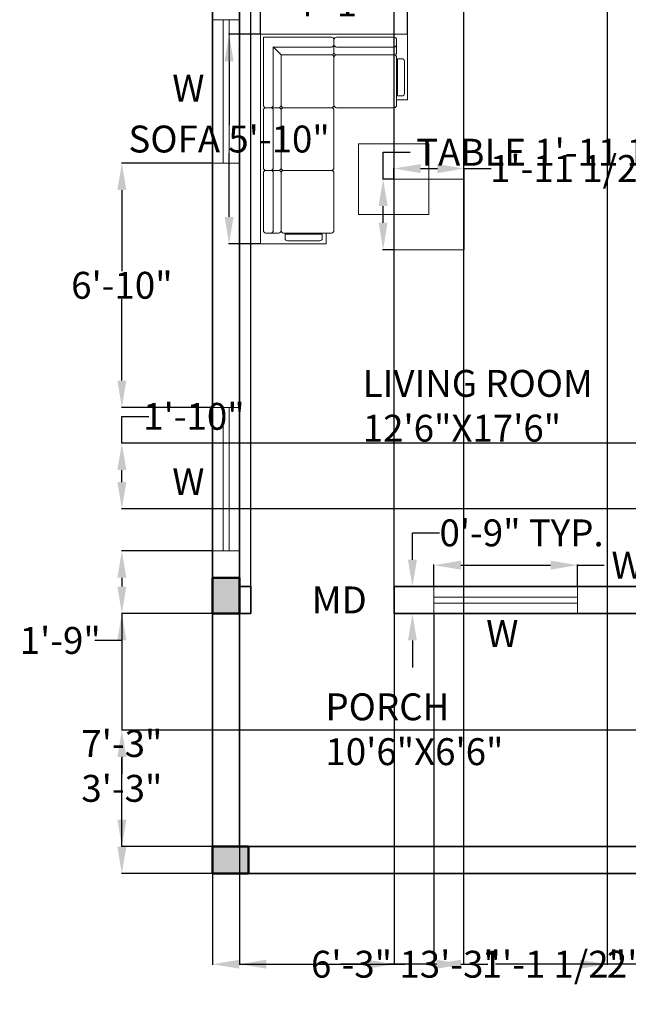
# Model space of a CAD drawing. Units: inches. Extents: x 113 to 575, y 111 to 799.
# Tile 1 of 4: x 113 to 317, y 111 to 441. Entities that reach past the tile are written whole.
import ezdxf

# ---------------------------------------------------------------- set-up
doc = ezdxf.new("R2010")
doc.units = ezdxf.units.IN
doc.header["$MEASUREMENT"] = 0
for name, color, linetype, lineweight in [('A-ANNO-DIMS', 2, 'Continuous', 18), ('A-ANNO-TEXT', 7, 'Continuous', 18), ('A-AREA-IDEN', 7, 'Continuous', 25), ('A-COLS', 7, 'Continuous', 50), ('A-COLS-PATT', 252, 'Continuous', 13), ('A-FURN', 8, 'Continuous', 18), ('A-GLAZ', 4, 'Continuous', 18), ('A-WALL', 7, 'Continuous', 35)]:
    doc.layers.add(name, color=color, linetype=linetype, lineweight=lineweight)
doc.styles.get("Standard").update_dxf_attribs({"font": 'arial.ttf'})
doc.dimstyles.get("Standard").update_dxf_attribs({"dimtxt": 9, "dimasz": 9, "dimexe": 0.18, "dimexo": 0.0625, "dimgap": 0.09, "dimtad": 0, "dimtih": 1, "dimtoh": 1, "dimdec": 0, "dimzin": 0, "dimdsep": 46, "dimlunit": 3, "dimtxsty": 'Standard', "dimcen": 0.09, "dimadec": 0, "dimazin": 0, "dimtfac": 1, "dimtdec": 0, "dimtofl": 0, "dimtmove": 0, "dimatfit": 3, "dimfxl": 1, "dimtolj": 1, "dimtzin": 0, "dimarcsym": 0})

# ---------------------------------------------------------------- blocks, each defined once
blk = doc.blocks.new('ММ318 1500х2140')
for p, q in [((-1390, 0), (-2140, 0)), ((-2140, 0), (-2140, -750)), ((-750, 0), (-1390, 0)), ((0, 0), (-750, 0)), ((0, 0), (0, -670)), ((-1415, -30), (-2110, -30)), ((-2110, -30), (-2110, -725)), ((-1390, -55), (-1390, -185)), ((-1390, -185), (-1390, -55)), ((-775, -30), (-1365, -30)), ((-750, -55), (-750, -185)), ((-750, -185), (-750, -55)), ((-135, -30), (-725, -30)), ((-110, -185), (-110, -55)), ((-2010, -135), (-2010, -725)), ((-1930, -210), (-2007, -132)), ((-1415, -130), (-2005, -130)), ((-2005, -130), (-2005, -130)), ((-775, -130), (-1365, -130)), ((-135, -130), (-725, -130)), ((-1930, -210), (-1415, -210)), ((-1930, -725), (-1930, -210)), ((-1390, -235), (-1390, -725)), ((-100, -250), (-55, -250)), ((-100, -250), (-100, -630)), ((-30, -275), (-30, -605)), ((-110, -670), (0, -670)), ((-100, -630), (-55, -630)), ((-2140, -1500), (-2140, -750)), ((-2110, -1365), (-2110, -775)), ((-2085, -750), (-1955, -750)), ((-2085, -750), (-1955, -750)), ((-2010, -1365), (-2010, -775)), ((-1415, -750), (-1905, -750)), ((-1955, -1390), (-2085, -1390)), ((-1890, -1400), (-1890, -1445)), ((-1890, -1400), (-1510, -1400)), ((-1510, -1400), (-1510, -1445)), ((-1470, -1390), (-1470, -1500)), ((-2140, -1500), (-1470, -1500)), ((-1865, -1470), (-1535, -1470))]:
    blk.add_line(p, q)
for points in [[(-1365, -210), (-775, -210, -0.414214), (-750, -235), (-750, -725, -0.414214), (-775, -750), (-1365, -750, -0.414214), (-1390, -725), (-1390, -235, -0.414214)], [(-725, -210), (-135, -210, -0.414214), (-110, -235), (-110, -725, -0.414214), (-135, -750), (-725, -750, -0.414214), (-750, -725), (-750, -235, -0.414214)], [(-1930, -775), (-1930, -1365, 0.414214), (-1905, -1390), (-1415, -1390, 0.414214), (-1390, -1365), (-1390, -775, 0.414214), (-1415, -750), (-1905, -750, 0.414214)]]:
    blk.add_lwpolyline(points, format="xyb", close=True)
for centre, start, end in [((-1415, -55), 0, 90), ((-1365, -55), 90, 180), ((-775, -55), 0, 90), ((-725, -55), 90, 180), ((-135, -55), 0, 90), ((-2005, -105), 256.9481, 270), ((-2035, -135), 0, 13.0519), ((-1415, -105), 270, 0), ((-1415, -185), 270, 0), ((-1365, -105), 180, 270), ((-1365, -185), 180, 270), ((-775, -105), 270, 0), ((-775, -185), 270, 0), ((-725, -105), 180, 270), ((-725, -185), 180, 270), ((-135, -105), 270, 0), ((-135, -185), 270, 0), ((-1415, -235), 0, 90), ((-55, -275), 0, 90), ((-55, -605), 270, 0), ((-2085, -725), 180, 270), ((-2085, -775), 90, 180), ((-2035, -725), 270, 0), ((-2035, -775), 0, 90), ((-1955, -725), 270, 0), ((-1955, -775), 0, 90), ((-1905, -725), 180, 270), ((-1415, -725), 270, 0), ((-2085, -1365), 180, 270), ((-2035, -1365), 270, 0), ((-1955, -1365), 270, 0), ((-1865, -1445), 180, 270), ((-1535, -1445), 270, 0)]:
    blk.add_arc(centre, 25, start, end)
blk = doc.blocks.new('ММ108 600х600')
blk.add_lwpolyline([(-600, 0), (0, 0), (0, -600), (-600, -600)], close=True)
blk = doc.blocks.new('WIN-48IN')
for p, q in [((0, 9), (0, 0)), ((48, 9), (48, 0)), ((0, 5.5), (48, 5.5)), ((0, 3.5), (48, 3.5))]:
    blk.add_line(p, q)
blk = doc.blocks.new('*D10')
at = {"layer": 'A-ANNO-DIMS', "color": 0, "lineweight": -2, "transparency": 16777216}
for p, q in [((251.58, 250.88), (251.58, 258.19)), ((260.58, 258.01), (290.58, 258.01)), ((299.58, 250.88), (299.58, 258.19)), ((299.58, 258.01), (308.58, 258.01))]:
    blk.add_line(p, q, dxfattribs=at)
at = {"layer": 'A-ANNO-DIMS', "color": 0, "transparency": 16777216}
for points in [[(260.58, 259.51), (260.58, 256.51), (251.58, 258.01)], [(290.58, 259.51), (290.58, 256.51), (299.58, 258.01)]]:
    blk.add_solid(points, dxfattribs=at)
at = {"layer": 'Defpoints', "color": 0, "transparency": 16777216}
for p in [(299.58, 258.01), (251.58, 250.81), (299.58, 250.81)]:
    blk.add_point(p, dxfattribs=at)
at = {"layer": 'A-ANNO-DIMS', "color": 0, "transparency": 16777216, "insert": (365.61, 258.01), "char_height": 9, "attachment_point": 5}
blk.add_mtext('\\A1;WINDOW 4\'-0" TYP.', dxfattribs=at)
blk = doc.blocks.new('*D11')
at = {"layer": 'A-ANNO-DIMS', "color": 0, "lineweight": -2, "transparency": 16777216}
for p, q in [((244.38, 259.81), (244.38, 268.81)), ((244.38, 268.81), (253.38, 268.81)), ((251.52, 250.81), (244.2, 250.81)), ((251.52, 241.81), (244.2, 241.81)), ((244.38, 232.81), (244.38, 223.81))]:
    blk.add_line(p, q, dxfattribs=at)
at = {"layer": 'A-ANNO-DIMS', "color": 0, "transparency": 16777216}
for points in [[(242.88, 259.81), (245.88, 259.81), (244.38, 250.81)], [(242.88, 232.81), (245.88, 232.81), (244.38, 241.81)]]:
    blk.add_solid(points, dxfattribs=at)
at = {"layer": 'Defpoints', "color": 0, "transparency": 16777216}
for p in [(244.38, 250.81), (251.58, 250.81), (251.58, 241.81)]:
    blk.add_point(p, dxfattribs=at)
at = {"layer": 'A-ANNO-DIMS', "color": 0, "transparency": 16777216, "insert": (280.9, 268.81), "char_height": 9, "attachment_point": 5}
blk.add_mtext('\\A1;0\'-9" TYP.', dxfattribs=at)
blk = doc.blocks.new('*D16')
at = {"layer": 'A-ANNO-DIMS', "color": 0, "lineweight": -2, "transparency": 16777216}
for p, q in [((234.56, 387.2), (234.56, 396.2)), ((234.56, 396.2), (243.56, 396.2)), ((238.04, 387.2), (234.38, 387.2)), ((234.56, 372.58), (234.56, 378.2)), ((238.04, 363.58), (234.38, 363.58))]:
    blk.add_line(p, q, dxfattribs=at)
at = {"layer": 'A-ANNO-DIMS', "color": 0, "transparency": 16777216}
for points in [[(233.06, 378.2), (236.06, 378.2), (234.56, 387.2)], [(233.06, 372.58), (236.06, 372.58), (234.56, 363.58)]]:
    blk.add_solid(points, dxfattribs=at)
at = {"layer": 'Defpoints', "color": 0, "transparency": 16777216}
for p in [(234.56, 387.2), (238.1, 387.2), (238.1, 363.58)]:
    blk.add_point(p, dxfattribs=at)
at = {"layer": 'A-ANNO-DIMS', "color": 0, "transparency": 16777216, "insert": (306.83, 396.2), "char_height": 9, "attachment_point": 5}
blk.add_mtext('\\A1;TABLE 1\'-11 1/2" TYP.', dxfattribs=at)
blk = doc.blocks.new('*D17')
at = {"layer": 'A-ANNO-DIMS', "color": 0, "lineweight": -2, "transparency": 16777216}
for p, q in [((238.1, 387.26), (238.1, 390.92)), ((247.1, 390.74), (252.72, 390.74)), ((261.72, 387.26), (261.72, 390.92)), ((261.72, 390.74), (270.72, 390.74))]:
    blk.add_line(p, q, dxfattribs=at)
at = {"layer": 'A-ANNO-DIMS', "color": 0, "transparency": 16777216}
for points in [[(247.1, 392.24), (247.1, 389.24), (238.1, 390.74)], [(252.72, 392.24), (252.72, 389.24), (261.72, 390.74)]]:
    blk.add_solid(points, dxfattribs=at)
at = {"layer": 'Defpoints', "color": 0, "transparency": 16777216}
for p in [(261.72, 390.74), (238.1, 387.2), (261.72, 387.2)]:
    blk.add_point(p, dxfattribs=at)
at = {"layer": 'A-ANNO-DIMS', "color": 0, "transparency": 16777216, "insert": (311.8, 390.74), "char_height": 9, "attachment_point": 5}
blk.add_mtext('\\A1;1\'-11 1/2" TYP.', dxfattribs=at)
blk = doc.blocks.new('*D20')
at = {"layer": 'A-ANNO-DIMS', "color": 0, "lineweight": -2, "transparency": 16777216}
for p, q in [((193.48, 435.68), (182.84, 435.68)), ((183.02, 426.68), (183.02, 405.37)), ((183.02, 374.56), (183.02, 395.87)), ((193.48, 365.56), (182.84, 365.56))]:
    blk.add_line(p, q, dxfattribs=at)
at = {"layer": 'A-ANNO-DIMS', "color": 0, "transparency": 16777216}
for points in [[(181.52, 426.68), (184.52, 426.68), (183.02, 435.68)], [(181.52, 374.56), (184.52, 374.56), (183.02, 365.56)]]:
    blk.add_solid(points, dxfattribs=at)
at = {"layer": 'Defpoints', "color": 0, "transparency": 16777216}
for p in [(193.54, 435.68), (183.02, 365.56), (193.54, 365.56)]:
    blk.add_point(p, dxfattribs=at)
at = {"layer": 'A-ANNO-DIMS', "color": 0, "transparency": 16777216, "insert": (183.02, 400.62), "char_height": 9, "attachment_point": 5}
blk.add_mtext('\\A1;SOFA 5\'-10"', dxfattribs=at)
blk = doc.blocks.new('*D21')
at = {"layer": 'A-ANNO-DIMS', "color": 0, "lineweight": -2, "transparency": 16777216}
for p, q in [((193.54, 435.74), (193.54, 446.38)), ((202.54, 446.2), (205.88, 446.2)), ((233.68, 446.2), (230.35, 446.2)), ((242.68, 435.74), (242.68, 446.38))]:
    blk.add_line(p, q, dxfattribs=at)
at = {"layer": 'A-ANNO-DIMS', "color": 0, "transparency": 16777216}
for points in [[(202.54, 447.7), (202.54, 444.7), (193.54, 446.2)], [(233.68, 447.7), (233.68, 444.7), (242.68, 446.2)]]:
    blk.add_solid(points, dxfattribs=at)
at = {"layer": 'Defpoints', "color": 0, "transparency": 16777216}
for p in [(193.54, 446.2), (193.54, 435.68), (242.68, 435.68)]:
    blk.add_point(p, dxfattribs=at)
at = {"layer": 'A-ANNO-DIMS', "color": 0, "transparency": 16777216, "insert": (218.11, 446.2), "char_height": 9, "attachment_point": 5}
blk.add_mtext('\\A1;4\'-1"', dxfattribs=at)
blk = doc.blocks.new('*D22')
at = {"layer": 'A-ANNO-DIMS', "color": 0, "lineweight": -2, "transparency": 16777216}
for p, q in [((177.49, 154.75), (177.49, 124.27)), ((336.49, 154.75), (336.49, 124.27)), ((186.49, 124.45), (241.87, 124.45)), ((327.49, 124.45), (272.12, 124.45))]:
    blk.add_line(p, q, dxfattribs=at)
at = {"layer": 'A-ANNO-DIMS', "color": 0, "transparency": 16777216}
for points in [[(186.49, 125.95), (186.49, 122.95), (177.49, 124.45)], [(327.49, 125.95), (327.49, 122.95), (336.49, 124.45)]]:
    blk.add_solid(points, dxfattribs=at)
at = {"layer": 'Defpoints', "color": 0, "transparency": 16777216}
for p in [(177.49, 154.81), (336.49, 154.81), (336.49, 124.45)]:
    blk.add_point(p, dxfattribs=at)
at = {"layer": 'A-ANNO-DIMS', "color": 0, "transparency": 16777216, "insert": (256.99, 124.45), "char_height": 9, "attachment_point": 5}
blk.add_mtext('\\A1;13\'-3"', dxfattribs=at)
blk = doc.blocks.new('*D25')
at = {"layer": 'A-ANNO-DIMS', "color": 0, "lineweight": -2, "transparency": 16777216}
for p, q in [((336.43, 202.81), (146.96, 202.81)), ((147.14, 193.81), (147.14, 188)), ((147.14, 172.81), (147.14, 178.62)), ((336.43, 163.81), (146.96, 163.81))]:
    blk.add_line(p, q, dxfattribs=at)
at = {"layer": 'A-ANNO-DIMS', "color": 0, "transparency": 16777216}
for points in [[(145.64, 193.81), (148.64, 193.81), (147.14, 202.81)], [(145.64, 172.81), (148.64, 172.81), (147.14, 163.81)]]:
    blk.add_solid(points, dxfattribs=at)
at = {"layer": 'Defpoints', "color": 0, "transparency": 16777216}
for p in [(147.14, 202.81), (336.49, 202.81), (336.49, 163.81)]:
    blk.add_point(p, dxfattribs=at)
at = {"layer": 'A-ANNO-DIMS', "color": 0, "transparency": 16777216, "insert": (147.14, 183.31), "char_height": 9, "attachment_point": 5}
blk.add_mtext('\\A1;3\'-3"', dxfattribs=at)
blk = doc.blocks.new('*D28')
at = {"layer": 'A-ANNO-DIMS', "color": 0, "lineweight": -2, "transparency": 16777216}
for p, q in [((190.28, 250.88), (190.28, 785.35)), ((199.28, 785.17), (202.05, 785.17)), ((229.28, 785.17), (226.51, 785.17)), ((238.28, 250.88), (238.28, 785.35))]:
    blk.add_line(p, q, dxfattribs=at)
at = {"layer": 'A-ANNO-DIMS', "color": 0, "transparency": 16777216}
for points in [[(199.28, 786.67), (199.28, 783.67), (190.28, 785.17)], [(229.28, 786.67), (229.28, 783.67), (238.28, 785.17)]]:
    blk.add_solid(points, dxfattribs=at)
at = {"layer": 'Defpoints', "color": 0, "transparency": 16777216}
for p in [(238.28, 785.17), (190.28, 250.81), (238.28, 250.81)]:
    blk.add_point(p, dxfattribs=at)
at = {"layer": 'A-ANNO-DIMS', "color": 0, "transparency": 16777216, "insert": (214.28, 785.17), "char_height": 9, "attachment_point": 5}
blk.add_mtext('\\A1;4\'-0"', dxfattribs=at)
blk = doc.blocks.new('*D33')
at = {"layer": 'A-ANNO-DIMS', "color": 0, "lineweight": -2, "transparency": 16777216}
for p, q in [((147.14, 298.81), (147.14, 307.81)), ((147.14, 307.81), (156.14, 307.81)), ((398.43, 298.81), (146.96, 298.81)), ((147.14, 285.81), (147.14, 289.81)), ((398.43, 276.81), (146.96, 276.81))]:
    blk.add_line(p, q, dxfattribs=at)
at = {"layer": 'A-ANNO-DIMS', "color": 0, "transparency": 16777216}
for points in [[(145.64, 289.81), (148.64, 289.81), (147.14, 298.81)], [(145.64, 285.81), (148.64, 285.81), (147.14, 276.81)]]:
    blk.add_solid(points, dxfattribs=at)
at = {"layer": 'Defpoints', "color": 0, "transparency": 16777216}
for p in [(147.14, 298.81), (398.49, 298.81), (398.49, 276.81)]:
    blk.add_point(p, dxfattribs=at)
at = {"layer": 'A-ANNO-DIMS', "color": 0, "transparency": 16777216, "insert": (171.26, 307.81), "char_height": 9, "attachment_point": 5}
blk.add_mtext('\\A1;1\'-10"', dxfattribs=at)
blk = doc.blocks.new('*D34')
at = {"layer": 'A-ANNO-DIMS', "color": 0, "lineweight": -2, "transparency": 16777216}
for p, q in [((177.43, 262.78), (146.96, 262.78)), ((147.14, 253.78), (147.14, 250.81)), ((177.43, 241.81), (146.96, 241.81)), ((147.14, 241.81), (147.14, 232.81)), ((147.14, 232.81), (138.14, 232.81))]:
    blk.add_line(p, q, dxfattribs=at)
at = {"layer": 'A-ANNO-DIMS', "color": 0, "transparency": 16777216}
for points in [[(145.64, 253.78), (148.64, 253.78), (147.14, 262.78)], [(145.64, 250.81), (148.64, 250.81), (147.14, 241.81)]]:
    blk.add_solid(points, dxfattribs=at)
at = {"layer": 'Defpoints', "color": 0, "transparency": 16777216}
for p in [(177.49, 262.78), (147.14, 241.81), (177.49, 241.81)]:
    blk.add_point(p, dxfattribs=at)
at = {"layer": 'A-ANNO-DIMS', "color": 0, "transparency": 16777216, "insert": (126.51, 232.81), "char_height": 9, "attachment_point": 5}
blk.add_mtext('\\A1;1\'-9"', dxfattribs=at)
blk = doc.blocks.new('*D35')
at = {"layer": 'A-ANNO-DIMS', "color": 0, "lineweight": -2, "transparency": 16777216}
for p, q in [((177.43, 392.56), (146.96, 392.56)), ((147.14, 383.56), (147.14, 356.36)), ((147.14, 319.78), (147.14, 346.99)), ((177.43, 310.78), (146.96, 310.78))]:
    blk.add_line(p, q, dxfattribs=at)
at = {"layer": 'A-ANNO-DIMS', "color": 0, "transparency": 16777216}
for points in [[(145.64, 383.56), (148.64, 383.56), (147.14, 392.56)], [(145.64, 319.78), (148.64, 319.78), (147.14, 310.78)]]:
    blk.add_solid(points, dxfattribs=at)
at = {"layer": 'Defpoints', "color": 0, "transparency": 16777216}
for p in [(147.14, 392.56), (177.49, 392.56), (177.49, 310.78)]:
    blk.add_point(p, dxfattribs=at)
at = {"layer": 'A-ANNO-DIMS', "color": 0, "transparency": 16777216, "insert": (147.14, 351.67), "char_height": 9, "attachment_point": 5}
blk.add_mtext('\\A1;6\'-10"', dxfattribs=at)
blk = doc.blocks.new('*D44')
at = {"layer": 'A-ANNO-DIMS', "color": 0, "lineweight": -2, "transparency": 16777216}
for p, q in [((238.28, 241.75), (238.28, 124.27)), ((251.58, 241.75), (251.58, 124.27)), ((229.28, 124.45), (220.28, 124.45)), ((260.58, 124.45), (269.58, 124.45))]:
    blk.add_line(p, q, dxfattribs=at)
at = {"layer": 'A-ANNO-DIMS', "color": 0, "transparency": 16777216}
for points in [[(229.28, 125.95), (229.28, 122.95), (238.28, 124.45)], [(260.58, 125.95), (260.58, 122.95), (251.58, 124.45)]]:
    blk.add_solid(points, dxfattribs=at)
at = {"layer": 'Defpoints', "color": 0, "transparency": 16777216}
for p in [(238.28, 241.81), (251.58, 241.81), (251.58, 124.45)]:
    blk.add_point(p, dxfattribs=at)
at = {"layer": 'A-ANNO-DIMS', "color": 0, "transparency": 16777216, "insert": (291.69, 124.45), "char_height": 9, "attachment_point": 5}
blk.add_mtext('\\A1;1\'-1 1/2"', dxfattribs=at)
blk = doc.blocks.new('*D48')
at = {"layer": 'A-ANNO-DIMS', "color": 0, "lineweight": -2, "transparency": 16777216}
for p, q in [((186.49, 592.75), (186.49, 124.27)), ((261.49, 592.75), (261.49, 124.27)), ((195.49, 124.45), (211.92, 124.45)), ((252.49, 124.45), (236.07, 124.45))]:
    blk.add_line(p, q, dxfattribs=at)
at = {"layer": 'A-ANNO-DIMS', "color": 0, "transparency": 16777216}
for points in [[(195.49, 125.95), (195.49, 122.95), (186.49, 124.45)], [(252.49, 125.95), (252.49, 122.95), (261.49, 124.45)]]:
    blk.add_solid(points, dxfattribs=at)
at = {"layer": 'Defpoints', "color": 0, "transparency": 16777216}
for p in [(186.49, 592.81), (261.49, 592.81), (261.49, 124.45)]:
    blk.add_point(p, dxfattribs=at)
at = {"layer": 'A-ANNO-DIMS', "color": 0, "transparency": 16777216, "insert": (223.99, 124.45), "char_height": 9, "attachment_point": 5}
blk.add_mtext('\\A1;6\'-3"', dxfattribs=at)
blk = doc.blocks.new('*D49')
at = {"layer": 'A-ANNO-DIMS', "color": 0, "lineweight": -2, "transparency": 16777216}
for p, q in [((309.494828, 592.750317), (309.494828, 124.273067)), ((336.494828, 592.750317), (336.494828, 124.273067)), ((300.494828, 124.453067), (291.494828, 124.453067)), ((345.494828, 124.453067), (354.494828, 124.453067))]:
    blk.add_line(p, q, dxfattribs=at)
at = {"layer": 'A-ANNO-DIMS', "color": 0, "transparency": 16777216}
for points in [[(300.494828, 125.953067), (300.494828, 122.953067), (309.494828, 124.453067)], [(345.494828, 125.953067), (345.494828, 122.953067), (336.494828, 124.453067)]]:
    blk.add_solid(points, dxfattribs=at)
at = {"layer": 'Defpoints', "color": 0, "transparency": 16777216}
for p in [(309.494828, 592.812817), (336.494828, 592.812817), (336.494828, 124.453067)]:
    blk.add_point(p, dxfattribs=at)
at = {"layer": 'A-ANNO-DIMS', "color": 0, "transparency": 16777216, "insert": (322.994828, 124.453067), "char_height": 9, "attachment_point": 5}
blk.add_mtext('\\A1;2\'-3"', dxfattribs=at)
blk = doc.blocks.new('*D52')
at = {"layer": 'A-ANNO-DIMS', "color": 0, "lineweight": -2, "transparency": 16777216}
for p, q in [((177.43, 241.81), (146.96, 241.81)), ((147.14, 232.81), (147.14, 203)), ((147.14, 163.81), (147.14, 193.62)), ((177.43, 154.81), (146.96, 154.81))]:
    blk.add_line(p, q, dxfattribs=at)
at = {"layer": 'A-ANNO-DIMS', "color": 0, "transparency": 16777216}
for points in [[(145.64, 232.81), (148.64, 232.81), (147.14, 241.81)], [(145.64, 163.81), (148.64, 163.81), (147.14, 154.81)]]:
    blk.add_solid(points, dxfattribs=at)
at = {"layer": 'Defpoints', "color": 0, "transparency": 16777216}
for p in [(147.14, 241.81), (177.49, 241.81), (177.49, 154.81)]:
    blk.add_point(p, dxfattribs=at)
at = {"layer": 'A-ANNO-DIMS', "color": 0, "transparency": 16777216, "insert": (147.14, 198.31), "char_height": 9, "attachment_point": 5}
blk.add_mtext('\\A1;7\'-3"', dxfattribs=at)
blk = doc.blocks.new('*D53')
at = {"layer": 'A-ANNO-DIMS', "color": 0, "lineweight": -2, "transparency": 16777216}
for p, q in [((177.49, 785.17), (168.49, 785.17)), ((186.49, 250.88), (186.49, 785.35)), ((190.28, 250.88), (190.28, 785.35)), ((199.28, 785.17), (208.28, 785.17))]:
    blk.add_line(p, q, dxfattribs=at)
at = {"layer": 'A-ANNO-DIMS', "color": 0, "transparency": 16777216}
for points in [[(177.49, 786.67), (177.49, 783.67), (186.49, 785.17)], [(199.28, 786.67), (199.28, 783.67), (190.28, 785.17)]]:
    blk.add_solid(points, dxfattribs=at)
at = {"layer": 'Defpoints', "color": 0, "transparency": 16777216}
for p in [(190.28, 785.17), (186.49, 250.81), (190.28, 250.81)]:
    blk.add_point(p, dxfattribs=at)
at = {"layer": 'A-ANNO-DIMS', "color": 0, "transparency": 16777216, "insert": (220.33, 785.17), "char_height": 9, "attachment_point": 5}
blk.add_mtext('\\A1;0\'-4"', dxfattribs=at)

msp = doc.modelspace()

# ---------------------------------------------------------------- hatches: boundary and pattern name
at = {"layer": 'A-COLS-PATT'}
h = msp.add_hatch(color=256, dxfattribs=at)
h.dxf.hatch_style = 1
h.paths.add_polyline_path([(186.49, 754.81), (177.49, 754.81), (177.49, 742.81), (186.49, 742.81)])
h.paths.add_polyline_path([(345.49, 754.81), (336.49, 754.81), (336.49, 742.81), (345.49, 742.81)])
h.paths.add_polyline_path([(489.49, 754.81), (480.49, 754.81), (480.49, 742.81), (489.49, 742.81)])
h.paths.add_polyline_path([(489.49, 601.81), (480.49, 601.81), (480.49, 589.81), (489.49, 589.81)])
h.paths.add_polyline_path([(345.49, 604.81), (336.49, 604.81), (336.49, 592.81), (345.49, 592.81)])
h.paths.add_polyline_path([(186.49, 604.81), (177.49, 604.81), (177.49, 592.81), (186.49, 592.81)])
h.paths.add_polyline_path([(186.49, 472.81), (177.49, 472.81), (177.49, 460.81), (186.49, 460.81)])
h.paths.add_polyline_path([(345.49, 469.81), (336.49, 469.81), (336.49, 457.81), (345.49, 457.81)])
h.paths.add_polyline_path([(489.49, 469.81), (480.49, 469.81), (480.49, 457.81), (489.49, 457.81)])
h.paths.add_polyline_path([(186.49, 253.81), (177.49, 253.81), (177.49, 241.81), (186.49, 241.81)])
h.paths.add_polyline_path([(345.49, 253.81), (336.49, 253.81), (336.49, 241.81), (345.49, 241.81)])
h.paths.add_polyline_path([(489.49, 253.81), (480.49, 253.81), (480.49, 241.81), (489.49, 241.81)])
h.paths.add_polyline_path([(489.49, 163.81), (477.49, 163.81), (477.49, 154.81), (489.49, 154.81)])
h.paths.add_polyline_path([(348.49, 163.81), (336.49, 163.81), (336.49, 154.81), (348.49, 154.81)])
h.paths.add_polyline_path([(189.49, 163.81), (177.49, 163.81), (177.49, 154.81), (189.49, 154.81)])

# ---------------------------------------------------------------- linework, layer by layer
at = {"layer": 'A-COLS'}
for points in [[(177.49, 253.81), (186.49, 253.81), (186.49, 241.81), (177.49, 241.81)], [(177.49, 154.81), (177.49, 163.81), (189.49, 163.81), (189.49, 154.81)]]:
    msp.add_lwpolyline(points, close=True, dxfattribs=at)
at = {"layer": 'A-WALL'}
for p, q in [((177.49, 154.81), (177.49, 754.81)), ((186.49, 163.81), (186.49, 592.81)), ((186.49, 250.81), (190.28, 250.81)), ((190.28, 250.81), (190.28, 241.81)), ((238.28, 250.81), (238.28, 241.81)), ((238.28, 250.81), (336.49, 250.81)), ((186.49, 241.81), (190.28, 241.81)), ((238.28, 241.81), (480.49, 241.81)), ((480.49, 163.81), (186.49, 163.81)), ((489.49, 154.81), (177.49, 154.81))]:
    msp.add_line(p, q, dxfattribs=at)

# ---------------------------------------------------------------- block references
at = {"layer": 'A-FURN', "xscale": -0.0327636075053148, "yscale": 0.0327636075053148, "zscale": 0.0327636075053148, "rotation": 90}
msp.add_blockref('ММ318 1500х2140', (193.54, 365.56), dxfattribs=at)
at = {"layer": 'A-FURN', "xscale": 0.0393700787401575, "yscale": 0.0393700787401575, "zscale": 0.0393700787401575}
for p in [(249.91, 399.01), (261.72, 387.2)]:
    msp.add_blockref('ММ108 600х600', p, dxfattribs=at)
at = {"layer": 'A-GLAZ', "rotation": 90.00000000000011}
for p in [(186.49, 392.56), (186.49, 262.79)]:
    msp.add_blockref('WIN-48IN', p, dxfattribs=at)
at = {"layer": 'A-GLAZ'}
msp.add_blockref('WIN-48IN', (251.58, 241.81), dxfattribs=at)

# ---------------------------------------------------------------- texts
at = {"layer": 'A-ANNO-TEXT', "char_height": 9, "attachment_point": 1}
for s, insert in [('W', (164, 422.16)), ('W', (164, 290.44)), ('MD', (210.69, 250.87)), ('W', (269.06, 239.6))]:
    msp.add_mtext_dynamic_manual_height_columns(s, width=17.4228, gutter_width=1, heights=[0], dxfattribs=dict(at, insert=insert))
at = {"layer": 'A-AREA-IDEN', "char_height": 9, "attachment_point": 1}
for s, insert in [('LIVING ROOM\\P12\'6"X17\'6"', (227.74, 323.34)), ('PORCH\\P10\'6"X6\'6"', (215.26, 215.09))]:
    msp.add_mtext_dynamic_manual_height_columns(s, width=130.397, gutter_width=1, heights=[0], dxfattribs=dict(at, insert=insert))

# ---------------------------------------------------------------- dimensions: what is measured, and where the dimension line sits
at = {"layer": 'A-ANNO-DIMS'}
for base, p1, p2, picture, middle in [((190.28, 785.17), (186.49, 250.81), (190.28, 250.81), '*D53', (220.33, 785.17)), ((238.28, 785.17), (190.28, 250.81), (238.28, 250.81), '*D28', (214.28, 785.17)), ((261.49, 124.45), (186.49, 592.81), (261.49, 592.81), '*D48', (223.99, 124.45)), ((336.49, 124.45), (309.49, 592.81), (336.49, 592.81), '*D49', (322.99, 124.45)), ((251.58, 124.45), (238.28, 241.81), (251.58, 241.81), '*D44', (291.69, 124.45)), ((336.49, 124.45), (177.49, 154.81), (336.49, 154.81), '*D22', (256.99, 124.45))]:
    dim = msp.add_linear_dim(base=base, p1=p1, p2=p2, dimstyle='Standard', override={"dimdec": 1, "dimlfac": 1, "dimrnd": 0, "dimzin": 1, "dimdsep": 46, "dimlunit": 4, "dimfrac": 2}, dxfattribs=at)
    dim.commit()
    dim.dimension.update_dxf_attribs({"geometry": picture, "text_midpoint": middle})
for base, p1, p2, angle, picture, middle in [((193.54, 446.2), (242.68, 435.68), (193.54, 435.68), 180, '*D21', (218.11, 446.2)), ((147.14, 392.56), (177.49, 310.78), (177.49, 392.56), 90, '*D35', (147.14, 351.67)), ((147.14, 298.81), (398.49, 276.81), (398.49, 298.81), 90, '*D33', (171.26, 307.81)), ((147.14, 241.81), (177.49, 262.78), (177.49, 241.81), 90, '*D34', (126.51, 232.81)), ((147.14, 241.81), (177.49, 154.81), (177.49, 241.81), 90, '*D52', (147.14, 198.31)), ((147.14, 202.81), (336.49, 163.81), (336.49, 202.81), 90, '*D25', (147.14, 183.31))]:
    dim = msp.add_linear_dim(base=base, p1=p1, p2=p2, angle=angle, dimstyle='Standard', override={"dimdec": 1, "dimlfac": 1, "dimrnd": 0, "dimzin": 1, "dimdsep": 46, "dimlunit": 4, "dimfrac": 2}, dxfattribs=at)
    dim.commit()
    dim.dimension.update_dxf_attribs({"geometry": picture, "text_midpoint": middle})
for base, p1, p2, angle, text, picture, middle in [((183.02, 365.56), (193.54, 435.68), (193.54, 365.56), 270, 'SOFA <>', '*D20', (183.02, 400.62)), ((234.56, 387.2), (238.1, 363.58), (238.1, 387.2), 90, 'TABLE <> TYP.', '*D16', (306.83, 396.2)), ((244.38, 250.81), (251.58, 241.81), (251.58, 250.81), 90, '<> TYP.', '*D11', (280.9, 268.81))]:
    dim = msp.add_linear_dim(base=base, p1=p1, p2=p2, angle=angle, text=text, dimstyle='Standard', override={"dimdec": 1, "dimlfac": 1, "dimrnd": 0, "dimzin": 1, "dimdsep": 46, "dimlunit": 4, "dimfrac": 2}, dxfattribs=at)
    dim.commit()
    dim.dimension.update_dxf_attribs({"geometry": picture, "text_midpoint": middle})
for base, p1, p2, text, picture, middle in [((261.72, 390.74), (238.1, 387.2), (261.72, 387.2), '<> TYP.', '*D17', (311.8, 390.74)), ((299.58, 258.01), (251.58, 250.81), (299.58, 250.81), 'WINDOW <> TYP.', '*D10', (365.61, 258.01))]:
    dim = msp.add_linear_dim(base=base, p1=p1, p2=p2, text=text, dimstyle='Standard', override={"dimdec": 1, "dimlfac": 1, "dimrnd": 0, "dimzin": 1, "dimdsep": 46, "dimlunit": 4, "dimfrac": 2}, dxfattribs=at)
    dim.commit()
    dim.dimension.update_dxf_attribs({"geometry": picture, "text_midpoint": middle})

doc.saveas('drawing.dxf')
